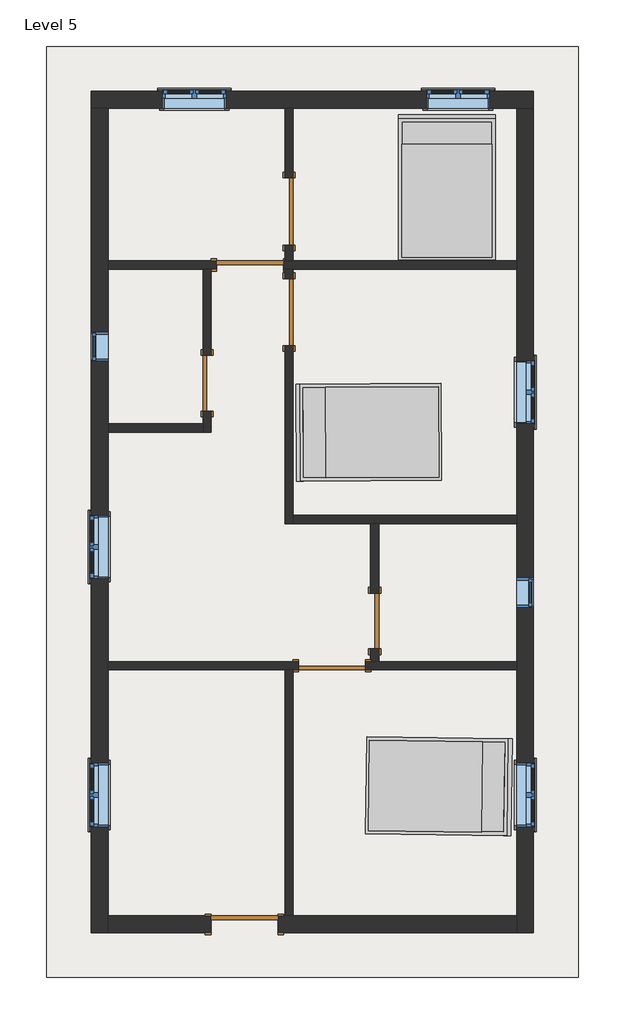
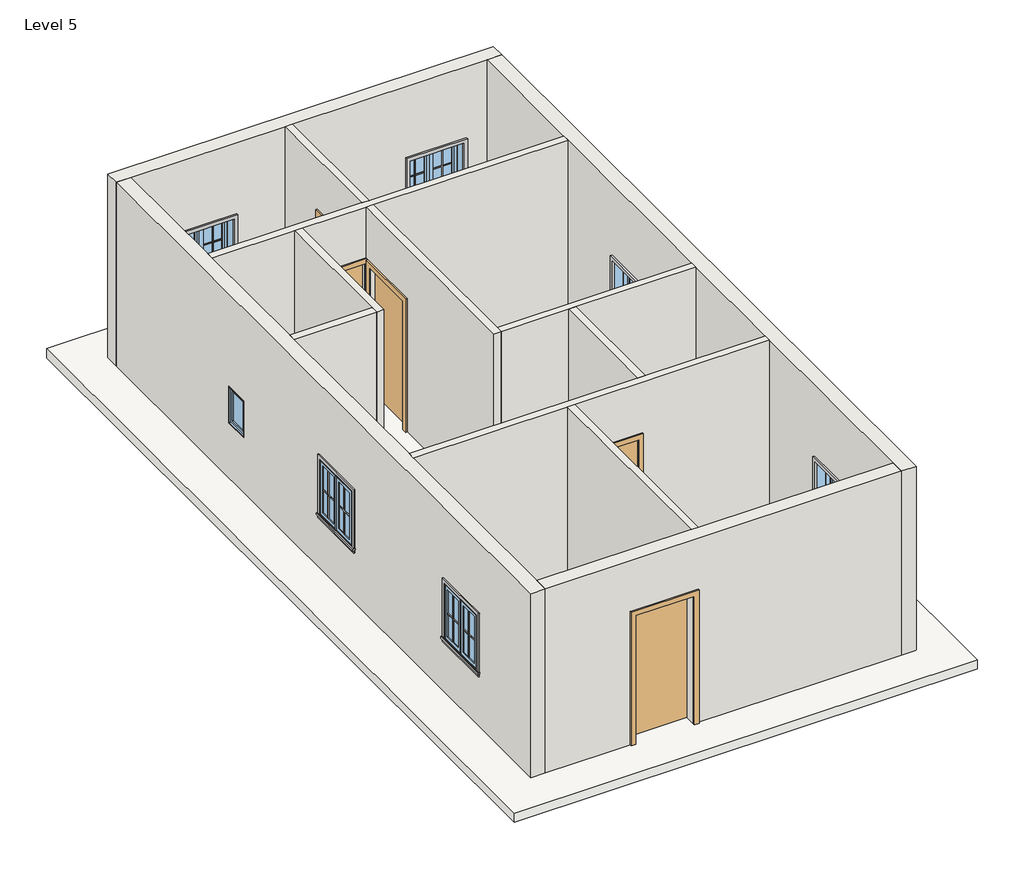
# One storey, incomplete: 24 proxies, 12 walls, 8 windows, 7 doors, 3 furniture elements, 1 roof.
"""IFC4 building model written with IfcOpenShell, lengths in millimetres."""

from ifc_helpers import new_model, si_unit, frame, origin, place, context, project, spatial, polyline, outline, extrude, faceted_brep, transform, mapped, element, save
from components import muntin_pattern_2x2_muntin_pattern_2x2_b3fe6957, muntin_pattern_2x2_muntin_pattern_2x2_3e0ecaf2, trim_window_exterior_flat_with_sill_41619996, trim_window_interior_flat_picture_frame_51c85655, door_d8f5dbb5, door_f2b275c1, door_e5f9f3c4, door_305aa2a5, door_0ca8825f, bed_17739_bed_17739_15c61121, window_aa618e30, window_339605e1

model = new_model("IFC4")

# Units and contexts
model_context = context("Model", 3, world=origin())
ifc_project = project(units=[si_unit("LENGTHUNIT", "METRE", prefix="MILLI")], contexts=[model_context])

# Site, building, storey
site = spatial("IfcSite", under=ifc_project)
building = spatial("IfcBuilding", under=site)
storey = spatial("IfcBuildingStorey", under=building, Name="Level 5", Elevation=9601.2)

# Proxies
placement = place(None, origin())
muntin_pattern_2x2_muntin_pattern_2x2_shape = muntin_pattern_2x2_muntin_pattern_2x2_b3fe6957(model_context)
element("IfcBuildingElementProxy", 1, Name="Muntin Pattern_2x2 : Muntin Pattern_2x2", ObjectType="Muntin Pattern_2x2 : Muntin Pattern_2x2", at=placement, inside=storey, context=model_context, shape_type="MappedRepresentation", body=[
    mapped(muntin_pattern_2x2_muntin_pattern_2x2_shape, transform((517.9959916, 6415.1185985, 10585.45), x_axis=(1.0, 0.0, 0.0), y_axis=(0.0, 1.0, 0.0), z_axis=(0.0, 0.0, 1.0))),
])
element("IfcBuildingElementProxy", 2, Name="Muntin Pattern_2x2 : Muntin Pattern_2x2", ObjectType="Muntin Pattern_2x2 : Muntin Pattern_2x2", at=placement, inside=storey, context=model_context, shape_type="MappedRepresentation", body=[
    mapped(muntin_pattern_2x2_muntin_pattern_2x2_shape, transform((-3079.2790084, 6415.1185985, 10585.45), x_axis=(1.0, 0.0, 0.0), y_axis=(0.0, 1.0, 0.0), z_axis=(0.0, 0.0, 1.0))),
])
element("IfcBuildingElementProxy", 3, Name="Muntin Pattern_2x2 : Muntin Pattern_2x2", ObjectType="Muntin Pattern_2x2 : Muntin Pattern_2x2", at=placement, inside=storey, context=model_context, shape_type="MappedRepresentation", body=[
    mapped(muntin_pattern_2x2_muntin_pattern_2x2_shape, transform((1751.4834916, 2536.8560985, 10585.45), x_axis=(0.0, -1.0, 0.0), y_axis=(1.0, 0.0, 0.0), z_axis=(0.0, 0.0, 1.0))),
])
element("IfcBuildingElementProxy", 4, Name="Muntin Pattern_2x2 : Muntin Pattern_2x2", ObjectType="Muntin Pattern_2x2 : Muntin Pattern_2x2", at=placement, inside=storey, context=model_context, shape_type="MappedRepresentation", body=[
    mapped(muntin_pattern_2x2_muntin_pattern_2x2_shape, transform((-4261.9665084, 0.0310985, 10585.45), x_axis=(0.0, 1.0, 0.0), y_axis=(-1.0, 0.0, 0.0), z_axis=(0.0, 0.0, 1.0))),
])
element("IfcBuildingElementProxy", 5, Name="Muntin Pattern_2x2 : Muntin Pattern_2x2", ObjectType="Muntin Pattern_2x2 : Muntin Pattern_2x2", at=placement, inside=storey, context=model_context, shape_type="MappedRepresentation", body=[
    mapped(muntin_pattern_2x2_muntin_pattern_2x2_shape, transform((-4261.9665084, -3381.3439015, 10585.45), x_axis=(0.0, 1.0, 0.0), y_axis=(-1.0, 0.0, 0.0), z_axis=(0.0, 0.0, 1.0))),
])
element("IfcBuildingElementProxy", 6, Name="Muntin Pattern_2x2 : Muntin Pattern_2x2", ObjectType="Muntin Pattern_2x2 : Muntin Pattern_2x2", at=placement, inside=storey, context=model_context, shape_type="MappedRepresentation", body=[
    mapped(muntin_pattern_2x2_muntin_pattern_2x2_shape, transform((1751.4834916, -2952.7189015, 10585.45), x_axis=(0.0, -1.0, 0.0), y_axis=(1.0, 0.0, 0.0), z_axis=(0.0, 0.0, 1.0))),
])
muntin_pattern_2x2_muntin_pattern_2x2_2_shape = muntin_pattern_2x2_muntin_pattern_2x2_3e0ecaf2(model_context)
element("IfcBuildingElementProxy", 7, Name="Muntin Pattern_2x2 : Muntin Pattern_2x2", ObjectType="Muntin Pattern_2x2 : Muntin Pattern_2x2", at=placement, inside=storey, context=model_context, shape_type="MappedRepresentation", body=[
    mapped(muntin_pattern_2x2_muntin_pattern_2x2_2_shape, transform((946.6209916, 6415.1185985, 10585.45), x_axis=(-1.0, 0.0, 0.0), y_axis=(0.0, -1.0, 0.0), z_axis=(0.0, 0.0, 1.0))),
])
element("IfcBuildingElementProxy", 8, Name="Muntin Pattern_2x2 : Muntin Pattern_2x2", ObjectType="Muntin Pattern_2x2 : Muntin Pattern_2x2", at=placement, inside=storey, context=model_context, shape_type="MappedRepresentation", body=[
    mapped(muntin_pattern_2x2_muntin_pattern_2x2_2_shape, transform((-2650.6540084, 6415.1185985, 10585.45), x_axis=(-1.0, 0.0, 0.0), y_axis=(0.0, -1.0, 0.0), z_axis=(0.0, 0.0, 1.0))),
])
element("IfcBuildingElementProxy", 9, Name="Muntin Pattern_2x2 : Muntin Pattern_2x2", ObjectType="Muntin Pattern_2x2 : Muntin Pattern_2x2", at=placement, inside=storey, context=model_context, shape_type="MappedRepresentation", body=[
    mapped(muntin_pattern_2x2_muntin_pattern_2x2_2_shape, transform((1751.4834916, 2108.2310985, 10585.45), x_axis=(0.0, 1.0, 0.0), y_axis=(-1.0, 0.0, 0.0), z_axis=(0.0, 0.0, 1.0))),
])
element("IfcBuildingElementProxy", 10, Name="Muntin Pattern_2x2 : Muntin Pattern_2x2", ObjectType="Muntin Pattern_2x2 : Muntin Pattern_2x2", at=placement, inside=storey, context=model_context, shape_type="MappedRepresentation", body=[
    mapped(muntin_pattern_2x2_muntin_pattern_2x2_2_shape, transform((-4261.9665084, 428.6560985, 10585.45), x_axis=(0.0, -1.0, 0.0), y_axis=(1.0, 0.0, 0.0), z_axis=(0.0, 0.0, 1.0))),
])
element("IfcBuildingElementProxy", 11, Name="Muntin Pattern_2x2 : Muntin Pattern_2x2", ObjectType="Muntin Pattern_2x2 : Muntin Pattern_2x2", at=placement, inside=storey, context=model_context, shape_type="MappedRepresentation", body=[
    mapped(muntin_pattern_2x2_muntin_pattern_2x2_2_shape, transform((-4261.9665084, -2952.7189015, 10585.45), x_axis=(0.0, -1.0, 0.0), y_axis=(1.0, 0.0, 0.0), z_axis=(0.0, 0.0, 1.0))),
])
element("IfcBuildingElementProxy", 12, Name="Muntin Pattern_2x2 : Muntin Pattern_2x2", ObjectType="Muntin Pattern_2x2 : Muntin Pattern_2x2", at=placement, inside=storey, context=model_context, shape_type="MappedRepresentation", body=[
    mapped(muntin_pattern_2x2_muntin_pattern_2x2_2_shape, transform((1751.4834916, -3381.3439015, 10585.45), x_axis=(0.0, 1.0, 0.0), y_axis=(-1.0, 0.0, 0.0), z_axis=(0.0, 0.0, 1.0))),
])
trim_window_exterior_flat_with_sill_shape = trim_window_exterior_flat_with_sill_41619996(model_context)
element("IfcBuildingElementProxy", 13, Name="Trim-Window-Exterior-Flat : with Sill", ObjectType="Trim-Window-Exterior-Flat : with Sill", at=placement, inside=storey, context=model_context, shape_type="MappedRepresentation", body=[
    mapped(trim_window_exterior_flat_with_sill_shape, transform((732.3084916, 6424.6435985, 11430.0), x_axis=(-1.0, 0.0, 0.0), y_axis=(0.0, 0.0, 1.0), z_axis=(0.0, 1.0, 0.0))),
])
element("IfcBuildingElementProxy", 14, Name="Trim-Window-Exterior-Flat : with Sill", ObjectType="Trim-Window-Exterior-Flat : with Sill", at=placement, inside=storey, context=model_context, shape_type="MappedRepresentation", body=[
    mapped(trim_window_exterior_flat_with_sill_shape, transform((-2864.9665084, 6424.6435985, 11430.0), x_axis=(-1.0, 0.0, 0.0), y_axis=(0.0, 0.0, 1.0), z_axis=(0.0, 1.0, 0.0))),
])
element("IfcBuildingElementProxy", 15, Name="Trim-Window-Exterior-Flat : with Sill", ObjectType="Trim-Window-Exterior-Flat : with Sill", at=placement, inside=storey, context=model_context, shape_type="MappedRepresentation", body=[
    mapped(trim_window_exterior_flat_with_sill_shape, transform((1761.0084916, 2322.5435985, 11430.0), x_axis=(0.0, 1.0, 0.0), y_axis=(0.0, 0.0, 1.0), z_axis=(1.0, 0.0, 0.0))),
])
element("IfcBuildingElementProxy", 16, Name="Trim-Window-Exterior-Flat : with Sill", ObjectType="Trim-Window-Exterior-Flat : with Sill", at=placement, inside=storey, context=model_context, shape_type="MappedRepresentation", body=[
    mapped(trim_window_exterior_flat_with_sill_shape, transform((-4271.4915084, 214.3435985, 11430.0), x_axis=(0.0, -1.0, 0.0), y_axis=(0.0, 0.0, 1.0), z_axis=(-1.0, 0.0, 0.0))),
])
element("IfcBuildingElementProxy", 17, Name="Trim-Window-Exterior-Flat : with Sill", ObjectType="Trim-Window-Exterior-Flat : with Sill", at=placement, inside=storey, context=model_context, shape_type="MappedRepresentation", body=[
    mapped(trim_window_exterior_flat_with_sill_shape, transform((-4271.4915084, -3167.0314015, 11430.0), x_axis=(0.0, -1.0, 0.0), y_axis=(0.0, 0.0, 1.0), z_axis=(-1.0, 0.0, 0.0))),
])
element("IfcBuildingElementProxy", 18, Name="Trim-Window-Exterior-Flat : with Sill", ObjectType="Trim-Window-Exterior-Flat : with Sill", at=placement, inside=storey, context=model_context, shape_type="MappedRepresentation", body=[
    mapped(trim_window_exterior_flat_with_sill_shape, transform((1761.0084916, -3167.0314015, 11430.0), x_axis=(0.0, 1.0, 0.0), y_axis=(0.0, 0.0, 1.0), z_axis=(1.0, 0.0, 0.0))),
])
trim_window_interior_flat_picture_frame_shape = trim_window_interior_flat_picture_frame_51c85655(model_context)
element("IfcBuildingElementProxy", 19, Name="Trim-Window-Interior-Flat : Picture Frame", ObjectType="Trim-Window-Interior-Flat : Picture Frame", at=placement, inside=storey, context=model_context, shape_type="MappedRepresentation", body=[
    mapped(trim_window_interior_flat_picture_frame_shape, transform((732.3084916, 6196.0435985, 11430.0), x_axis=(1.0, 0.0, 0.0), y_axis=(0.0, 0.0, 1.0), z_axis=(0.0, -1.0, 0.0))),
])
element("IfcBuildingElementProxy", 20, Name="Trim-Window-Interior-Flat : Picture Frame", ObjectType="Trim-Window-Interior-Flat : Picture Frame", at=placement, inside=storey, context=model_context, shape_type="MappedRepresentation", body=[
    mapped(trim_window_interior_flat_picture_frame_shape, transform((-2864.9665084, 6196.0435985, 11430.0), x_axis=(1.0, 0.0, 0.0), y_axis=(0.0, 0.0, 1.0), z_axis=(0.0, -1.0, 0.0))),
])
element("IfcBuildingElementProxy", 21, Name="Trim-Window-Interior-Flat : Picture Frame", ObjectType="Trim-Window-Interior-Flat : Picture Frame", at=placement, inside=storey, context=model_context, shape_type="MappedRepresentation", body=[
    mapped(trim_window_interior_flat_picture_frame_shape, transform((1532.4084916, 2322.5435985, 11430.0), x_axis=(0.0, -1.0, 0.0), y_axis=(0.0, 0.0, 1.0), z_axis=(-1.0, 0.0, 0.0))),
])
element("IfcBuildingElementProxy", 22, Name="Trim-Window-Interior-Flat : Picture Frame", ObjectType="Trim-Window-Interior-Flat : Picture Frame", at=placement, inside=storey, context=model_context, shape_type="MappedRepresentation", body=[
    mapped(trim_window_interior_flat_picture_frame_shape, transform((-4042.8915084, 214.3435985, 11430.0), x_axis=(0.0, 1.0, 0.0), y_axis=(0.0, 0.0, 1.0), z_axis=(1.0, 0.0, 0.0))),
])
element("IfcBuildingElementProxy", 23, Name="Trim-Window-Interior-Flat : Picture Frame", ObjectType="Trim-Window-Interior-Flat : Picture Frame", at=placement, inside=storey, context=model_context, shape_type="MappedRepresentation", body=[
    mapped(trim_window_interior_flat_picture_frame_shape, transform((-4042.8915084, -3167.0314015, 11430.0), x_axis=(0.0, 1.0, 0.0), y_axis=(0.0, 0.0, 1.0), z_axis=(1.0, 0.0, 0.0))),
])
element("IfcBuildingElementProxy", 24, Name="Trim-Window-Interior-Flat : Picture Frame", ObjectType="Trim-Window-Interior-Flat : Picture Frame", at=placement, inside=storey, context=model_context, shape_type="MappedRepresentation", body=[
    mapped(trim_window_interior_flat_picture_frame_shape, transform((1532.4084916, -3167.0314015, 11430.0), x_axis=(0.0, -1.0, 0.0), y_axis=(0.0, 0.0, 1.0), z_axis=(-1.0, 0.0, 0.0))),
])

# Doors
door_shape = door_d8f5dbb5(model_context)
element("IfcDoor", 25, ObjectType="Single-Flush : 30\" x 80\"", at=placement, inside=storey, context=model_context, shape_type="MappedRepresentation", body=[
    mapped(door_shape, transform((-404.3415084, -795.3064015, 9601.2), x_axis=(0.0, -1.0, 0.0), y_axis=(1.0, 0.0, 0.0), z_axis=(0.0, 0.0, 1.0))),
])
door_2_shape = door_f2b275c1(model_context)
element("IfcDoor", 26, ObjectType="Single-Flush : 30\" x 80\"", at=placement, inside=storey, context=model_context, shape_type="MappedRepresentation", body=[
    mapped(door_2_shape, transform((-2690.3415084, 2443.1935985, 9601.2), x_axis=(0.0, -1.0, 0.0), y_axis=(1.0, 0.0, 0.0), z_axis=(0.0, 0.0, 1.0))),
])
door_3_shape = door_e5f9f3c4(model_context)
element("IfcDoor", 27, ObjectType="Single-Flush : 36\" x 84\"", at=placement, inside=storey, context=model_context, shape_type="MappedRepresentation", body=[
    mapped(door_3_shape, transform((-2106.1415084, 4056.0935985, 9601.2), x_axis=(1.0, 0.0, 0.0), y_axis=(0.0, 1.0, 0.0), z_axis=(0.0, 0.0, 1.0))),
])
element("IfcDoor", 28, ObjectType="Single-Flush : 36\" x 84\"", at=placement, inside=storey, context=model_context, shape_type="MappedRepresentation", body=[
    mapped(door_3_shape, transform((-1572.7415084, 4786.3435985, 9601.2), x_axis=(0.0, -1.0, 0.0), y_axis=(1.0, 0.0, 0.0), z_axis=(0.0, 0.0, 1.0))),
])
element("IfcDoor", 29, ObjectType="Single-Flush : 36\" x 84\"", at=placement, inside=storey, context=model_context, shape_type="MappedRepresentation", body=[
    mapped(door_3_shape, transform((-988.5415084, -1404.9064015, 9601.2), x_axis=(-1.0, 0.0, 0.0), y_axis=(0.0, -1.0, 0.0), z_axis=(0.0, 0.0, 1.0))),
])
door_4_shape = door_305aa2a5(model_context)
element("IfcDoor", 30, ObjectType="Single-Flush : 36\" x 84\"", at=placement, inside=storey, context=model_context, shape_type="MappedRepresentation", body=[
    mapped(door_4_shape, transform((-1572.7415084, 3414.7435985, 9601.2), x_axis=(0.0, 1.0, 0.0), y_axis=(-1.0, 0.0, 0.0), z_axis=(0.0, 0.0, 1.0))),
])
door_5_shape = door_0ca8825f(model_context)
element("IfcDoor", 31, ObjectType="Single-Flush : 36\" x 84\"", at=placement, inside=storey, context=model_context, shape_type="MappedRepresentation", body=[
    mapped(door_5_shape, transform((-2182.3415084, -4929.1564015, 9601.2), x_axis=(1.0, 0.0, 0.0), y_axis=(0.0, 1.0, 0.0), z_axis=(0.0, 0.0, 1.0))),
])

# Furniture
bed_17739_bed_17739_shape = bed_17739_bed_17739_15c61121(model_context)
element("IfcFurniture", 32, ObjectType="Bed_17739 : Bed_17739", at=placement, inside=storey, context=model_context, shape_type="MappedRepresentation", body=[
    mapped(bed_17739_bed_17739_shape, transform((579.9084916, 5091.1435985, 9601.2), x_axis=(1.0, 0.0, 0.0), y_axis=(0.0, 1.0, 0.0), z_axis=(0.0, 0.0, 1.0))),
])
element("IfcFurniture", 33, ObjectType="Bed_17739 : Bed_17739", at=placement, inside=storey, context=model_context, shape_type="MappedRepresentation", body=[
    mapped(bed_17739_bed_17739_shape, transform((-461.4915084, 1776.4435985, 9601.2), x_axis=(-0.00529598194226197, 0.9999859761893001, 0.0), y_axis=(-0.9999859761893001, -0.00529598194226197, 0.0), z_axis=(0.0, 0.0, 1.0))),
])
element("IfcFurniture", 34, ObjectType="Bed_17739 : Bed_17739", at=placement, inside=storey, context=model_context, shape_type="MappedRepresentation", body=[
    mapped(bed_17739_bed_17739_shape, transform((445.2457081, -3048.1973462, 9601.2), x_axis=(-0.012781947661401841, -0.9999183075701641, 0.0), y_axis=(0.9999183075701641, -0.012781947661401841, 0.0), z_axis=(0.0, 0.0, 1.0))),
])

# Roof
element("IfcRoof", 35, ObjectType="Generic - 12\"", at=placement, inside=storey, context=model_context, shape_type="SweptSolid", body=[
    extrude(outline(polyline([(-4881.0915084, 7034.2435985), (2370.6084916, 7034.2435985), (2370.6084916, -5653.0564015), (-4881.0915084, -5653.0564015), (-4881.0915084, 7034.2435985)])), frame((0.0, 0.0, 9448.8), z_axis=(0.0, 0.0, 1.0), x_axis=(1.0, 0.0, 0.0)), (0.0, 0.0, 1.0), 152.4),
])

# Walls
element("IfcWall", 36, ObjectType="WALL4.5\"", at=placement, inside=storey, context=model_context, shape_type="Brep", body=[
    faceted_brep([(-1648.9415084, 3998.9435985, 11734.8), (-1648.9415084, 3998.9435985, 9601.2), (-1629.8915084, 3998.9435985, 9601.2), (-1515.5915084, 3998.9435985, 9601.2), (1532.4084916, 3998.9435985, 9601.2), (1532.4084916, 3998.9435985, 12649.2), (-1515.5915084, 3998.9435985, 12649.2), (-1629.8915084, 3998.9435985, 12649.2), (-2633.1915084, 3998.9435985, 12649.2), (-2747.4915084, 3998.9435985, 12649.2), (-4042.8915084, 3998.9435985, 12649.2), (-4042.8915084, 3998.9435985, 9601.2), (-2747.4915084, 3998.9435985, 9601.2), (-2633.1915084, 3998.9435985, 9601.2), (-2563.3415084, 3998.9435985, 9601.2), (-2563.3415084, 3998.9435985, 11734.8), (1532.4084916, 4113.2435985, 9601.2), (-1515.5915084, 4113.2435985, 9601.2), (-1629.8915084, 4113.2435985, 9601.2), (-1648.9415084, 4113.2435985, 9601.2), (-1648.9415084, 4113.2435985, 11734.8), (-2563.3415084, 4113.2435985, 11734.8), (-2563.3415084, 4113.2435985, 9601.2), (-4042.8915084, 4113.2435985, 9601.2), (-4042.8915084, 4113.2435985, 12649.2), (-1629.8915084, 4113.2435985, 12649.2), (-1515.5915084, 4113.2435985, 12649.2), (1532.4084916, 4113.2435985, 12649.2)], [[[0, 1, 2, 3, 4, 5, 6, 7, 8, 9, 10, 11, 12, 13, 14, 15]], [[16, 17, 18, 19, 20, 21, 22, 23, 24, 25, 26, 27]], [[4, 3, 2, 1, 19, 18, 17, 16]], [[14, 13, 12, 11, 23, 22]], [[5, 4, 16, 27]], [[11, 10, 24, 23]], [[20, 19, 1, 0]], [[21, 20, 0, 15]], [[22, 21, 15, 14]], [[10, 9, 8, 7, 6, 5, 27, 26, 25, 24]]]),
])
element("IfcWall", 37, ObjectType="WALL4.5\"", at=placement, inside=storey, context=model_context, shape_type="Brep", body=[
    faceted_brep([(-1629.8915084, 6196.0435985, 12649.2), (-1629.8915084, 6196.0435985, 9601.2), (-1629.8915084, 5243.5435985, 9601.2), (-1629.8915084, 5243.5435985, 11734.8), (-1629.8915084, 4329.1435985, 11734.8), (-1629.8915084, 4329.1435985, 9601.2), (-1629.8915084, 4113.2435985, 9601.2), (-1629.8915084, 4113.2435985, 12649.2), (-1515.5915084, 6196.0435985, 9601.2), (-1515.5915084, 6196.0435985, 12649.2), (-1515.5915084, 4113.2435985, 12649.2), (-1515.5915084, 4113.2435985, 9601.2), (-1515.5915084, 4329.1435985, 9601.2), (-1515.5915084, 4329.1435985, 11734.8), (-1515.5915084, 5243.5435985, 11734.8), (-1515.5915084, 5243.5435985, 9601.2)], [[[0, 1, 2, 3, 4, 5, 6, 7]], [[8, 9, 10, 11, 12, 13, 14, 15]], [[1, 8, 15, 2]], [[5, 12, 11, 6]], [[1, 0, 9, 8]], [[7, 6, 11, 10]], [[13, 12, 5, 4]], [[14, 13, 4, 3]], [[15, 14, 3, 2]], [[9, 0, 7, 10]]]),
    faceted_brep([(-1629.8915084, 531.8435985, 9601.2), (-1629.8915084, 531.8435985, 12649.2), (-1629.8915084, 3998.9435985, 12649.2), (-1629.8915084, 3998.9435985, 9601.2), (-1629.8915084, 3871.9435985, 9601.2), (-1629.8915084, 3871.9435985, 11734.8), (-1629.8915084, 2957.5435985, 11734.8), (-1629.8915084, 2957.5435985, 9601.2), (-1515.5915084, 531.8435985, 12649.2), (-1515.5915084, 531.8435985, 9601.2), (-1515.5915084, 646.1435985, 9601.2), (-1515.5915084, 2957.5435985, 9601.2), (-1515.5915084, 2957.5435985, 11734.8), (-1515.5915084, 3871.9435985, 11734.8), (-1515.5915084, 3871.9435985, 9601.2), (-1515.5915084, 3998.9435985, 9601.2), (-1515.5915084, 3998.9435985, 12649.2), (-1515.5915084, 646.1435985, 12649.2)], [[[0, 1, 2, 3, 4, 5, 6, 7]], [[8, 9, 10, 11, 12, 13, 14, 15, 16, 17]], [[9, 0, 7, 11, 10]], [[14, 4, 3, 15]], [[3, 2, 16, 15]], [[1, 0, 9, 8]], [[5, 4, 14, 13]], [[6, 5, 13, 12]], [[7, 6, 12, 11]], [[1, 8, 17, 16, 2]]]),
])
element("IfcWall", 38, ObjectType="WALL4.5\"", at=placement, inside=storey, context=model_context, shape_type="Brep", body=[
    faceted_brep([(-1515.5915084, 531.8435985, 9601.2), (-461.4915084, 531.8435985, 9601.2), (-347.1915084, 531.8435985, 9601.2), (1532.4084916, 531.8435985, 9601.2), (1532.4084916, 531.8435985, 12649.2), (-347.1915084, 531.8435985, 12649.2), (-461.4915084, 531.8435985, 12649.2), (-1515.5915084, 531.8435985, 12649.2), (-1515.5915084, 646.1435985, 9601.2), (-1515.5915084, 646.1435985, 12649.2), (1532.4084916, 646.1435985, 12649.2), (1532.4084916, 646.1435985, 9601.2)], [[[0, 1, 2, 3, 4, 5, 6, 7]], [[8, 9, 10, 11]], [[3, 2, 1, 0, 8, 11]], [[0, 7, 9, 8]], [[4, 3, 11, 10]], [[7, 6, 5, 4, 10, 9]]]),
])
element("IfcWall", 39, ObjectType="WALL4.5\"", at=placement, inside=storey, context=model_context, shape_type="Brep", body=[
    faceted_brep([(-2747.4915084, 2062.1935985, 11633.2), (-2747.4915084, 2062.1935985, 9601.2), (-2747.4915084, 1890.7435985, 9601.2), (-2747.4915084, 1776.4435985, 9601.2), (-2747.4915084, 1776.4435985, 12649.2), (-2747.4915084, 1890.7435985, 12649.2), (-2747.4915084, 3998.9435985, 12649.2), (-2747.4915084, 3998.9435985, 9601.2), (-2747.4915084, 2824.1935985, 9601.2), (-2747.4915084, 2824.1935985, 11633.2), (-2633.1915084, 1776.4435985, 9601.2), (-2633.1915084, 2062.1935985, 9601.2), (-2633.1915084, 2062.1935985, 11633.2), (-2633.1915084, 2824.1935985, 11633.2), (-2633.1915084, 2824.1935985, 9601.2), (-2633.1915084, 3998.9435985, 9601.2), (-2633.1915084, 3998.9435985, 12649.2), (-2633.1915084, 1776.4435985, 12649.2)], [[[0, 1, 2, 3, 4, 5, 6, 7, 8, 9]], [[10, 11, 12, 13, 14, 15, 16, 17]], [[8, 7, 15, 14]], [[3, 2, 1, 11, 10]], [[7, 6, 16, 15]], [[4, 3, 10, 17]], [[12, 11, 1, 0]], [[13, 12, 0, 9]], [[14, 13, 9, 8]], [[6, 5, 4, 17, 16]]]),
])
element("IfcWall", 40, ObjectType="WALL4.5\"", at=placement, inside=storey, context=model_context, shape_type="SweptSolid", body=[
    extrude(outline(polyline([(-2747.4915084, 1776.4435985), (-4042.8915084, 1776.4435985), (-4042.8915084, 1890.7435985), (-2747.4915084, 1890.7435985), (-2747.4915084, 1776.4435985)])), frame((0.0, 0.0, 9601.2), z_axis=(0.0, 0.0, 1.0), x_axis=(1.0, 0.0, 0.0)), (0.0, 0.0, 1.0), 3048.0),
])
element("IfcWall", 41, ObjectType="WALL4.5\"", at=placement, inside=storey, context=model_context, shape_type="SweptSolid", body=[
    extrude(outline(polyline([(-1176.3064015, 11633.2), (-1176.3064015, 9601.2), (-1347.7564015, 9601.2), (-1347.7564015, 12649.2), (531.8435985, 12649.2), (531.8435985, 9601.2), (-414.3064015, 9601.2), (-414.3064015, 11633.2), (-1176.3064015, 11633.2)])), frame((-461.4915084, 0.0, 0.0), z_axis=(1.0, 0.0, 0.0), x_axis=(0.0, 1.0, 0.0)), (0.0, 0.0, 1.0), 114.3),
])
element("IfcWall", 42, ObjectType="WALL4.5\"", at=placement, inside=storey, context=model_context, shape_type="Brep", body=[
    faceted_brep([(-4042.8915084, -1462.0564015, 9601.2), (-1629.8915084, -1462.0564015, 9601.2), (-1515.5915084, -1462.0564015, 9601.2), (-1445.7415084, -1462.0564015, 9601.2), (-1445.7415084, -1462.0564015, 11734.8), (-531.3415084, -1462.0564015, 11734.8), (-531.3415084, -1462.0564015, 9601.2), (1532.4084916, -1462.0564015, 9601.2), (1532.4084916, -1462.0564015, 12649.2), (-1515.5915084, -1462.0564015, 12649.2), (-1629.8915084, -1462.0564015, 12649.2), (-4042.8915084, -1462.0564015, 12649.2), (-1445.7415084, -1347.7564015, 11734.8), (-1445.7415084, -1347.7564015, 9601.2), (-4042.8915084, -1347.7564015, 9601.2), (-4042.8915084, -1347.7564015, 12649.2), (-461.4915084, -1347.7564015, 12649.2), (-347.1915084, -1347.7564015, 12649.2), (1532.4084916, -1347.7564015, 12649.2), (1532.4084916, -1347.7564015, 9601.2), (-347.1915084, -1347.7564015, 9601.2), (-461.4915084, -1347.7564015, 9601.2), (-531.3415084, -1347.7564015, 9601.2), (-531.3415084, -1347.7564015, 11734.8)], [[[0, 1, 2, 3, 4, 5, 6, 7, 8, 9, 10, 11]], [[12, 13, 14, 15, 16, 17, 18, 19, 20, 21, 22, 23]], [[14, 13, 3, 2, 1, 0]], [[22, 21, 20, 19, 7, 6]], [[8, 7, 19, 18]], [[0, 11, 15, 14]], [[4, 3, 13, 12]], [[5, 4, 12, 23]], [[6, 5, 23, 22]], [[11, 10, 9, 8, 18, 17, 16, 15]]]),
])
element("IfcWall", 43, ObjectType="WALL4.5\"", at=placement, inside=storey, context=model_context, shape_type="SweptSolid", body=[
    extrude(outline(polyline([(-1629.8915084, -4814.8564015), (-1629.8915084, -1462.0564015), (-1515.5915084, -1462.0564015), (-1515.5915084, -4814.8564015), (-1629.8915084, -4814.8564015)])), frame((0.0, 0.0, 9601.2), z_axis=(0.0, 0.0, 1.0), x_axis=(1.0, 0.0, 0.0)), (0.0, 0.0, 1.0), 3048.0),
])
element("IfcWall", 44, ObjectType="WALL9\"", at=placement, inside=storey, context=model_context, shape_type="Brep", body=[
    faceted_brep([(-4271.4915084, 6196.0435985, 9601.2), (-4042.8915084, 6196.0435985, 9601.2), (-1629.8915084, 6196.0435985, 9601.2), (-1515.5915084, 6196.0435985, 9601.2), (1532.4084916, 6196.0435985, 9601.2), (1761.0084916, 6196.0435985, 9601.2), (1761.0084916, 6196.0435985, 12649.2), (1532.4084916, 6196.0435985, 12649.2), (-1515.5915084, 6196.0435985, 12649.2), (-1629.8915084, 6196.0435985, 12649.2), (-4042.8915084, 6196.0435985, 12649.2), (-4271.4915084, 6196.0435985, 12649.2), (1164.1084916, 6196.0435985, 11430.0), (1164.1084916, 6196.0435985, 10515.6), (300.5084916, 6196.0435985, 10515.6), (300.5084916, 6196.0435985, 11430.0), (-2433.1665084, 6196.0435985, 11430.0), (-2433.1665084, 6196.0435985, 10515.6), (-3296.7665084, 6196.0435985, 10515.6), (-3296.7665084, 6196.0435985, 11430.0), (-4271.4915084, 6424.6435985, 9601.2), (-4271.4915084, 6424.6435985, 12649.2), (1761.0084916, 6424.6435985, 12649.2), (1761.0084916, 6424.6435985, 9601.2), (1164.1084916, 6424.6435985, 11430.0), (300.5084916, 6424.6435985, 11430.0), (300.5084916, 6424.6435985, 10515.6), (1164.1084916, 6424.6435985, 10515.6), (-2433.1665084, 6424.6435985, 11430.0), (-3296.7665084, 6424.6435985, 11430.0), (-3296.7665084, 6424.6435985, 10515.6), (-2433.1665084, 6424.6435985, 10515.6)], [[[0, 1, 2, 3, 4, 5, 6, 7, 8, 9, 10, 11], [12, 13, 14, 15], [16, 17, 18, 19]], [[20, 21, 22, 23], [24, 25, 26, 27], [28, 29, 30, 31]], [[5, 4, 3, 2, 1, 0, 20, 23]], [[6, 5, 23, 22]], [[0, 11, 21, 20]], [[13, 12, 24, 27]], [[14, 13, 27, 26]], [[15, 14, 26, 25]], [[12, 15, 25, 24]], [[17, 16, 28, 31]], [[18, 17, 31, 30]], [[19, 18, 30, 29]], [[16, 19, 29, 28]], [[11, 10, 9, 8, 7, 6, 22, 21]]]),
])
element("IfcWall", 45, ObjectType="WALL9\"", at=placement, inside=storey, context=model_context, shape_type="Brep", body=[
    faceted_brep([(1532.4084916, 6196.0435985, 9601.2), (1532.4084916, 4113.2435985, 9601.2), (1532.4084916, 3998.9435985, 9601.2), (1532.4084916, 646.1435985, 9601.2), (1532.4084916, 531.8435985, 9601.2), (1532.4084916, -1347.7564015, 9601.2), (1532.4084916, -1462.0564015, 9601.2), (1532.4084916, -4814.8564015, 9601.2), (1532.4084916, -5043.4564015, 9601.2), (1532.4084916, -5043.4564015, 12649.2), (1532.4084916, -4814.8564015, 12649.2), (1532.4084916, -1462.0564015, 12649.2), (1532.4084916, -1347.7564015, 12649.2), (1532.4084916, 531.8435985, 12649.2), (1532.4084916, 646.1435985, 12649.2), (1532.4084916, 3998.9435985, 12649.2), (1532.4084916, 4113.2435985, 12649.2), (1532.4084916, 6196.0435985, 12649.2), (1532.4084916, -611.1564015, 11125.2), (1532.4084916, -611.1564015, 10515.6), (1532.4084916, -204.7564015, 10515.6), (1532.4084916, -204.7564015, 11125.2), (1532.4084916, 1890.7435985, 11430.0), (1532.4084916, 1890.7435985, 10515.6), (1532.4084916, 2754.3435985, 10515.6), (1532.4084916, 2754.3435985, 11430.0), (1532.4084916, -3598.8314015, 11430.0), (1532.4084916, -3598.8314015, 10515.6), (1532.4084916, -2735.2314015, 10515.6), (1532.4084916, -2735.2314015, 11430.0), (1761.0084916, 6196.0435985, 9601.2), (1761.0084916, 6196.0435985, 12649.2), (1761.0084916, -5043.4564015, 12649.2), (1761.0084916, -5043.4564015, 9601.2), (1761.0084916, -611.1564015, 11125.2), (1761.0084916, -204.7564015, 11125.2), (1761.0084916, -204.7564015, 10515.6), (1761.0084916, -611.1564015, 10515.6), (1761.0084916, 1890.7435985, 11430.0), (1761.0084916, 2754.3435985, 11430.0), (1761.0084916, 2754.3435985, 10515.6), (1761.0084916, 1890.7435985, 10515.6), (1761.0084916, -3598.8314015, 11430.0), (1761.0084916, -2735.2314015, 11430.0), (1761.0084916, -2735.2314015, 10515.6), (1761.0084916, -3598.8314015, 10515.6)], [[[0, 1, 2, 3, 4, 5, 6, 7, 8, 9, 10, 11, 12, 13, 14, 15, 16, 17], [18, 19, 20, 21], [22, 23, 24, 25], [26, 27, 28, 29]], [[30, 31, 32, 33], [34, 35, 36, 37], [38, 39, 40, 41], [42, 43, 44, 45]], [[8, 7, 6, 5, 4, 3, 2, 1, 0, 30, 33]], [[0, 17, 31, 30]], [[9, 8, 33, 32]], [[19, 18, 34, 37]], [[20, 19, 37, 36]], [[21, 20, 36, 35]], [[18, 21, 35, 34]], [[23, 22, 38, 41]], [[24, 23, 41, 40]], [[25, 24, 40, 39]], [[22, 25, 39, 38]], [[27, 26, 42, 45]], [[28, 27, 45, 44]], [[29, 28, 44, 43]], [[26, 29, 43, 42]], [[17, 16, 15, 14, 13, 12, 11, 10, 9, 32, 31]]]),
])
element("IfcWall", 46, ObjectType="WALL9\"", at=placement, inside=storey, context=model_context, shape_type="Brep", body=[
    faceted_brep([(-4271.4915084, 6196.0435985, 9601.2), (-4271.4915084, -5043.4564015, 9601.2), (-4271.4915084, -5043.4564015, 12649.2), (-4271.4915084, 6196.0435985, 12649.2), (-4271.4915084, 3148.0435985, 11125.2), (-4271.4915084, 2741.6435985, 11125.2), (-4271.4915084, 2741.6435985, 10515.6), (-4271.4915084, 3148.0435985, 10515.6), (-4271.4915084, 646.1435985, 11430.0), (-4271.4915084, -217.4564015, 11430.0), (-4271.4915084, -217.4564015, 10515.6), (-4271.4915084, 646.1435985, 10515.6), (-4271.4915084, -2735.2314015, 11430.0), (-4271.4915084, -3598.8314015, 11430.0), (-4271.4915084, -3598.8314015, 10515.6), (-4271.4915084, -2735.2314015, 10515.6), (-4042.8915084, 6196.0435985, 9601.2), (-4042.8915084, 6196.0435985, 12649.2), (-4042.8915084, 4113.2435985, 12649.2), (-4042.8915084, 3998.9435985, 12649.2), (-4042.8915084, 1890.7435985, 12649.2), (-4042.8915084, 1776.4435985, 12649.2), (-4042.8915084, -1347.7564015, 12649.2), (-4042.8915084, -1462.0564015, 12649.2), (-4042.8915084, -4814.8564015, 12649.2), (-4042.8915084, -5043.4564015, 12649.2), (-4042.8915084, -5043.4564015, 9601.2), (-4042.8915084, -4814.8564015, 9601.2), (-4042.8915084, -1462.0564015, 9601.2), (-4042.8915084, -1347.7564015, 9601.2), (-4042.8915084, 1776.4435985, 9601.2), (-4042.8915084, 1890.7435985, 9601.2), (-4042.8915084, 3998.9435985, 9601.2), (-4042.8915084, 4113.2435985, 9601.2), (-4042.8915084, 3148.0435985, 11125.2), (-4042.8915084, 3148.0435985, 10515.6), (-4042.8915084, 2741.6435985, 10515.6), (-4042.8915084, 2741.6435985, 11125.2), (-4042.8915084, 646.1435985, 11430.0), (-4042.8915084, 646.1435985, 10515.6), (-4042.8915084, -217.4564015, 10515.6), (-4042.8915084, -217.4564015, 11430.0), (-4042.8915084, -2735.2314015, 11430.0), (-4042.8915084, -2735.2314015, 10515.6), (-4042.8915084, -3598.8314015, 10515.6), (-4042.8915084, -3598.8314015, 11430.0)], [[[0, 1, 2, 3], [4, 5, 6, 7], [8, 9, 10, 11], [12, 13, 14, 15]], [[16, 17, 18, 19, 20, 21, 22, 23, 24, 25, 26, 27, 28, 29, 30, 31, 32, 33], [34, 35, 36, 37], [38, 39, 40, 41], [42, 43, 44, 45]], [[1, 0, 16, 33, 32, 31, 30, 29, 28, 27, 26]], [[0, 3, 17, 16]], [[2, 1, 26, 25]], [[35, 34, 4, 7]], [[36, 35, 7, 6]], [[37, 36, 6, 5]], [[34, 37, 5, 4]], [[39, 38, 8, 11]], [[40, 39, 11, 10]], [[41, 40, 10, 9]], [[38, 41, 9, 8]], [[43, 42, 12, 15]], [[44, 43, 15, 14]], [[45, 44, 14, 13]], [[42, 45, 13, 12]], [[3, 2, 25, 24, 23, 22, 21, 20, 19, 18, 17]]]),
])
element("IfcWall", 47, ObjectType="WALL9\"", at=placement, inside=storey, context=model_context, shape_type="Brep", body=[
    faceted_brep([(-1725.1415084, -5043.4564015, 11734.8), (-1725.1415084, -5043.4564015, 9601.2), (1532.4084916, -5043.4564015, 9601.2), (1532.4084916, -5043.4564015, 12649.2), (-4042.8915084, -5043.4564015, 12649.2), (-4042.8915084, -5043.4564015, 9601.2), (-2639.5415084, -5043.4564015, 9601.2), (-2639.5415084, -5043.4564015, 11734.8), (1532.4084916, -4814.8564015, 9601.2), (-1515.5915084, -4814.8564015, 9601.2), (-1629.8915084, -4814.8564015, 9601.2), (-1725.1415084, -4814.8564015, 9601.2), (-1725.1415084, -4814.8564015, 11734.8), (-2639.5415084, -4814.8564015, 11734.8), (-2639.5415084, -4814.8564015, 9601.2), (-4042.8915084, -4814.8564015, 9601.2), (-4042.8915084, -4814.8564015, 12649.2), (-1629.8915084, -4814.8564015, 12649.2), (-1515.5915084, -4814.8564015, 12649.2), (1532.4084916, -4814.8564015, 12649.2)], [[[0, 1, 2, 3, 4, 5, 6, 7]], [[8, 9, 10, 11, 12, 13, 14, 15, 16, 17, 18, 19]], [[6, 5, 15, 14]], [[2, 1, 11, 10, 9, 8]], [[3, 2, 8, 19]], [[5, 4, 16, 15]], [[12, 11, 1, 0]], [[13, 12, 0, 7]], [[14, 13, 7, 6]], [[4, 3, 19, 18, 17, 16]]]),
])

# Windows
window_shape = window_aa618e30(model_context)
element("IfcWindow", 48, ObjectType="Fixed : 16\" x 24\"", at=placement, inside=storey, context=model_context, shape_type="MappedRepresentation", body=[
    mapped(window_shape, transform((1646.7084916, -446.0564015, 9601.2), x_axis=(0.0, -1.0, 0.0), y_axis=(1.0, 0.0, 0.0), z_axis=(0.0, 0.0, 1.0))),
])
element("IfcWindow", 49, ObjectType="Fixed : 16\" x 24\"", at=placement, inside=storey, context=model_context, shape_type="MappedRepresentation", body=[
    mapped(window_shape, transform((-4157.1915084, 2982.9435985, 9601.2), x_axis=(0.0, 1.0, 0.0), y_axis=(-1.0, 0.0, 0.0), z_axis=(0.0, 0.0, 1.0))),
])
window_2_shape = window_339605e1(model_context)
element("IfcWindow", 50, ObjectType="Window-Casement-Double : 34\" x 36\"", at=placement, inside=storey, context=model_context, shape_type="MappedRepresentation", body=[
    mapped(window_2_shape, transform((732.3084916, 6310.3435985, 9601.2), x_axis=(1.0, 0.0, 0.0), y_axis=(0.0, 1.0, 0.0), z_axis=(0.0, 0.0, 1.0))),
])
element("IfcWindow", 51, ObjectType="Window-Casement-Double : 34\" x 36\"", at=placement, inside=storey, context=model_context, shape_type="MappedRepresentation", body=[
    mapped(window_2_shape, transform((-2864.9665084, 6310.3435985, 9601.2), x_axis=(1.0, 0.0, 0.0), y_axis=(0.0, 1.0, 0.0), z_axis=(0.0, 0.0, 1.0))),
])
element("IfcWindow", 52, ObjectType="Window-Casement-Double : 34\" x 36\"", at=placement, inside=storey, context=model_context, shape_type="MappedRepresentation", body=[
    mapped(window_2_shape, transform((1646.7084916, 2322.5435985, 9601.2), x_axis=(0.0, -1.0, 0.0), y_axis=(1.0, 0.0, 0.0), z_axis=(0.0, 0.0, 1.0))),
])
element("IfcWindow", 53, ObjectType="Window-Casement-Double : 34\" x 36\"", at=placement, inside=storey, context=model_context, shape_type="MappedRepresentation", body=[
    mapped(window_2_shape, transform((-4157.1915084, 214.3435985, 9601.2), x_axis=(0.0, 1.0, 0.0), y_axis=(-1.0, 0.0, 0.0), z_axis=(0.0, 0.0, 1.0))),
])
element("IfcWindow", 54, ObjectType="Window-Casement-Double : 34\" x 36\"", at=placement, inside=storey, context=model_context, shape_type="MappedRepresentation", body=[
    mapped(window_2_shape, transform((-4157.1915084, -3167.0314015, 9601.2), x_axis=(0.0, 1.0, 0.0), y_axis=(-1.0, 0.0, 0.0), z_axis=(0.0, 0.0, 1.0))),
])
element("IfcWindow", 55, ObjectType="Window-Casement-Double : 34\" x 36\"", at=placement, inside=storey, context=model_context, shape_type="MappedRepresentation", body=[
    mapped(window_2_shape, transform((1646.7084916, -3167.0314015, 9601.2), x_axis=(0.0, -1.0, 0.0), y_axis=(1.0, 0.0, 0.0), z_axis=(0.0, 0.0, 1.0))),
])

save(model, "model.ifc")

# Revit data of these elements
# Type "Muntin Pattern_2x2 : Muntin Pattern_2x2"
#   Width [instance default] = 4' - 0"
#   Thickness = 0' - 0 1/2"
#   Height [instance default] = 4' - 0"
#   Distance = 0' - 0 3/4"
#   Interior Material [instance default] = none
#   Exterior Material [instance default] = none
#   Default Elevation = 0
# Type "Trim-Window-Exterior-Flat : with Sill"
#   Trim Width = 0' - 2 1/4"
#   Trim Thickness_Picture Frame = 0' - 1 1/4"
#   Trim Thickness_with Sill = 0' - 0 3/4"
#   Sill Thickness = 0' - 1 1/4"
#   Opening Width [instance default] = 2' - 0"
#   Opening Height [instance default] = 3' - 0"
#   Default Elevation = 4' - 0"
#   Sill = yes
#   Picture Frame = no
#   Trim Material [instance default] = none
# Type "Trim-Window-Interior-Flat : Picture Frame"
#   Trim Thickness_Picture Frame = 0' - 1 1/4"
#   Trim Width = 0' - 2 1/4"
#   Trim Thickness_with Sill = 0' - 0 3/4"
#   Sill Thickness = 0' - 1 1/4"
#   Opening Width [instance default] = 2' - 0"
#   Opening Height [instance default] = 3' - 0"
#   Default Elevation = 4' - 0"
#   Sill = no
#   Picture Frame = yes
#   Trim Material [instance default] = none
# Type "Single-Flush : 30\" x 80\""
#   Type Mark = "5"
#   Construction Type Id = "MDOOR"
#   Assembly Code = "C1020"
#   Analytic Construction = "Metal"
#   Thickness = 0' - 2"
#   Heat Transfer Coefficient (U) = 0.651978 BTU/(h·ft²·°F)
#   Height = 6' - 8"
#   Trim Projection Ext = 0' - 1"
#   Trim Projection Int = 0' - 1"
#   Trim Width = 0' - 3"
#   Width = 2' - 6"
#   Define Thermal Properties by = 1
#   Define Thermal Properties by = 1
#   Door Material = Door - Panel
#   Frame Material = Door - Frame
#   Visual Light Transmittance = 0
#   Solar Heat Gain Coefficient = 0
#   Function = (empty or 0)
#   Wall Closure = (empty or 0)
# Type "Single-Flush : 36\" x 84\""
#   Type Mark = "1"
#   Construction Type Id = "MDOOR"
#   Assembly Code = "C1020"
#   Analytic Construction = "Metal"
#   Thickness = 0' - 2"
#   Heat Transfer Coefficient (U) = 0.651978 BTU/(h·ft²·°F)
#   Height = 7' - 0"
#   Trim Projection Ext = 0' - 1"
#   Trim Projection Int = 0' - 1"
#   Trim Width = 0' - 3"
#   Width = 3' - 0"
#   Define Thermal Properties by = 1
#   Define Thermal Properties by = 1
#   Door Material = Door - Panel
#   Frame Material = Door - Frame
#   Visual Light Transmittance = 0
#   Solar Heat Gain Coefficient = 0
#   Function = (empty or 0)
#   Wall Closure = (empty or 0)
# Type "Bed_17739 : Bed_17739"
#   Default Elevation = 0
# Type "Generic - 12\""
#   Assembly Code = "B1020"
#   Layers, outside or top first: 0' - 6" no material (function 1)
# Type "WALL4.5\""
#   Assembly Code = "B2010"
#   Layers, outside or top first: 0' - 4 1/2" no material (function 1)
# Type "WALL9\""
#   Assembly Code = "B2010"
#   Layers, outside or top first: 0' - 9" no material (function 1)
# Type "Fixed : 16\" x 24\""
#   Type Mark = "4"
#   Construction Type Id = "GSP4R"
#   Assembly Code = "B2020100"
#   Analytic Construction = "1/8 in Pilkington single glazing"
#   Visual Light Transmittance = 0.9
#   Solar Heat Gain Coefficient = 0.78
#   Heat Transfer Coefficient (U) = 0.6496 BTU/(h·ft²·°F)
#   Height = 2' - 0"
#   Default Sill Height = 3' - 0"
#   Width = 1' - 4"
#   Window Inset = 0' - 0 3/4"
#   Define Thermal Properties by = 1
#   Define Thermal Properties by = 1
#   Glass Pane Material = Glass
#   Sash Material = Sash
#   Wall Closure = (empty or 0)
# Type "Window-Casement-Double : 34\" x 36\""
#   Type Mark = "14"
#   Fire Rating = "0.5h"
#   Assembly Code = "B2020100"
#   Analytic Construction = "Double glazing - domestic"
#   Frame Extension [instance default] = 0' - 0 1/4"
#   Window Inset [instance default] = 0' - 0"
#   Wall Thickness [instance default] = 0' - 6"
#   Interior Wall Closure [instance default] = 0' - 2 1/4"
#   Half Width = 1' - 5"
#   Visual Light Transmittance = 0.81
#   Thermal Resistance (R) = 1.8146 (h·ft²·°F)/BTU
#   Solar Heat Gain Coefficient = 0.76
#   Rough Width = 2' - 10 1/2"
#   Rough Height = 3' - 0 1/2"
#   Height = 3' - 0"
#   Heat Transfer Coefficient (U) = 0.5511 BTU/(h·ft²·°F)
#   Exterior Wall Closure [instance default] = 0' - 1 1/4"
#   Extension Jamb [instance default] = 0' - 2 1/4"
#   Default Sill Height = 3' - 0"
#   Width = 2' - 10"
#   Define Thermal Properties by = 0
#   Muntin Visibility = yes
#   Interior Trim Visibility [instance default] = yes
#   Exterior Trim Visibility [instance default] = yes
#   Extension Jamb Visibility [instance default] = yes
#   Interior Trim Material = Wood - Stained
#   Muntin Pattern = Muntin Pattern_2x2 : Muntin Pattern_2x2
#   Interior Trim = Trim-Window-Interior-Flat : Picture Frame
#   Interior Frame Material = Wood - Stained
#   Glass Panel Material = Glass
#   Exterior Trim Material = Clad - White
#   Exterior Trim = Trim-Window-Exterior-Flat : with Sill
#   Exterior Frame Material = Clad - White
#   Wall Closure = (empty or 0)
# Elements 1, 2, 3, 4, 5, 6, 7, 8, 9, 10, 11, 12 (IfcBuildingElementProxy, "Muntin Pattern_2x2 : Muntin Pattern_2x2")
#   Width = 0' - 11 5/8"
#   Height = 2' - 6 1/2"
#   Interior Material = Wood - Stained
#   Exterior Material = Clad - White
#   Phase Created = New Construction
#   Materials on its faces: "Clad - White", "Wood - Stained"
# Elements 13, 14, 15, 16, 17, 18 (IfcBuildingElementProxy, "Trim-Window-Exterior-Flat : with Sill")
#   Opening Width = 2' - 10"
#   Opening Height = 3' - 0"
#   Trim Material = Clad - White
#   Phase Created = New Construction
#   Materials on its faces: "Clad - White"
# Elements 19, 20, 21, 22, 23, 24 (IfcBuildingElementProxy, "Trim-Window-Interior-Flat : Picture Frame")
#   Opening Width = 2' - 10"
#   Opening Height = 3' - 0"
#   Trim Material = Wood - Stained
#   Phase Created = New Construction
#   Materials on its faces: "Wood - Stained"
# Elements 25, 26 (IfcDoor, "Single-Flush : 30\" x 80\"")
#   Phase Created = New Construction
#   Materials on its faces: "Door - Frame", "Door - Panel"
# Elements 27, 28, 29, 30, 31 (IfcDoor, "Single-Flush : 36\" x 84\"")
#   Phase Created = New Construction
#   Materials on its faces: "Door - Frame", "Door - Panel"
# Elements 32, 33, 34 (IfcFurniture, "Bed_17739 : Bed_17739")
#   Phase Created = New Construction
#   Materials on its faces: "legs", "sheets", "bed frame", "Blanket"
# Element 35 (IfcRoof, "Generic - 12\"")
#   built-in parameter 1001705 = 31.5 (stored number, unit not read)
#   built-in parameter 1001701 = -0.5 (stored number, unit not read)
#   built-in parameter 1001710 = 33615
#   Phase Created = New Construction
#   Materials on its faces: "Default Roof"
# Elements 36, 37, 38, 39, 40, 41, 42, 43 (IfcWall, "WALL4.5\"")
#   Top Offset = 0' - 0"
#   Base Offset = 0' - 0"
#   Unconnected Height = 10' - 0"
#   wall height = 10' - 0"
#   Phase Created = New Construction
#   Base Constraint = Level 5
#   Materials on its faces: "Default Wall"
# Elements 44, 45, 46, 47 (IfcWall, "WALL9\"")
#   Top Offset = 0' - 0"
#   Base Offset = 0' - 0"
#   Unconnected Height = 10' - 0"
#   wall height = 10' - 0"
#   Phase Created = New Construction
#   Base Constraint = Level 5
#   Materials on its faces: "Default Wall", "Brick, Common"
# Element 48 (IfcWindow, "Fixed : 16\" x 24\"")
#   Mark = "25"
#   Phase Created = New Construction
#   Materials on its faces: "Sash", "Glass"
# Element 49 (IfcWindow, "Fixed : 16\" x 24\"")
#   Mark = "26"
#   Phase Created = New Construction
#   Materials on its faces: "Sash", "Glass"
# Element 50 (IfcWindow, "Window-Casement-Double : 34\" x 36\"")
#   Mark = "27"
#   Window Inset = 0' - 0"
#   Interior Wall Closure = 0' - 2 1/4"
#   Frame Extension = 0' - 0 1/4"
#   Exterior Wall Closure = 0' - 1 1/4"
#   Interior Trim Visibility = yes
#   Exterior Trim Visibility = yes
#   Phase Created = New Construction
#   Materials on its faces: "Wood - Stained", "Glass", "Clad - White"
# Element 51 (IfcWindow, "Window-Casement-Double : 34\" x 36\"")
#   Mark = "28"
#   Window Inset = 0' - 0"
#   Interior Wall Closure = 0' - 2 1/4"
#   Frame Extension = 0' - 0 1/4"
#   Exterior Wall Closure = 0' - 1 1/4"
#   Interior Trim Visibility = yes
#   Exterior Trim Visibility = yes
#   Phase Created = New Construction
#   Materials on its faces: "Wood - Stained", "Glass", "Clad - White"
# Element 52 (IfcWindow, "Window-Casement-Double : 34\" x 36\"")
#   Mark = "29"
#   Window Inset = 0' - 0"
#   Interior Wall Closure = 0' - 2 1/4"
#   Frame Extension = 0' - 0 1/4"
#   Exterior Wall Closure = 0' - 1 1/4"
#   Interior Trim Visibility = yes
#   Exterior Trim Visibility = yes
#   Phase Created = New Construction
#   Materials on its faces: "Wood - Stained", "Glass", "Clad - White"
# Element 53 (IfcWindow, "Window-Casement-Double : 34\" x 36\"")
#   Mark = "30"
#   Window Inset = 0' - 0"
#   Interior Wall Closure = 0' - 2 1/4"
#   Frame Extension = 0' - 0 1/4"
#   Exterior Wall Closure = 0' - 1 1/4"
#   Interior Trim Visibility = yes
#   Exterior Trim Visibility = yes
#   Phase Created = New Construction
#   Materials on its faces: "Wood - Stained", "Glass", "Clad - White"
# Element 54 (IfcWindow, "Window-Casement-Double : 34\" x 36\"")
#   Mark = "31"
#   Window Inset = 0' - 0"
#   Interior Wall Closure = 0' - 2 1/4"
#   Frame Extension = 0' - 0 1/4"
#   Exterior Wall Closure = 0' - 1 1/4"
#   Interior Trim Visibility = yes
#   Exterior Trim Visibility = yes
#   Phase Created = New Construction
#   Materials on its faces: "Wood - Stained", "Glass", "Clad - White"
# Element 55 (IfcWindow, "Window-Casement-Double : 34\" x 36\"")
#   Mark = "32"
#   Window Inset = 0' - 0"
#   Interior Wall Closure = 0' - 2 1/4"
#   Frame Extension = 0' - 0 1/4"
#   Exterior Wall Closure = 0' - 1 1/4"
#   Interior Trim Visibility = yes
#   Exterior Trim Visibility = yes
#   Phase Created = New Construction
#   Materials on its faces: "Wood - Stained", "Glass", "Clad - White"
# Materials
#   "Door - Panel": class "Wood", colour RGB 210 159 95, transparency 0, Cost = 0
#   "Door - Frame": colour RGB 118 70 51, transparency 0, Cost = 0
#   "Glass": class "Glass", colour RGB 0 128 192, transparency 0.75, Description = "Soda Lime Glass", Cost = 0
#   "Sash": class "Wood", colour RGB 224 178 126, transparency 0, Cost = 0
#   "Wood - Stained": class "Wood", colour RGB 224 178 126, transparency 0, Cost = 0
#   "Clad - White": class "Wood", colour RGB 242 242 238, transparency 0, Cost = 0
#   "legs": colour RGB 90 73 37, transparency 0, Cost = 0
#   "sheets": colour RGB 200 195 176, transparency 0, Cost = 0
#   "bed frame": colour RGB 90 73 37, transparency 0, Cost = 0
#   "Blanket": class "System", colour RGB 59 0 1, transparency 0, Cost = 0
#   "Default Roof": colour RGB 88 101 114, transparency 0, Cost = 0
#   "Default Wall": colour RGB 128 128 128, transparency 0, Cost = 0
#   "Brick, Common": class "Masonry", colour RGB 170 98 104, transparency 0, Description = "Common brick", Cost = 0
